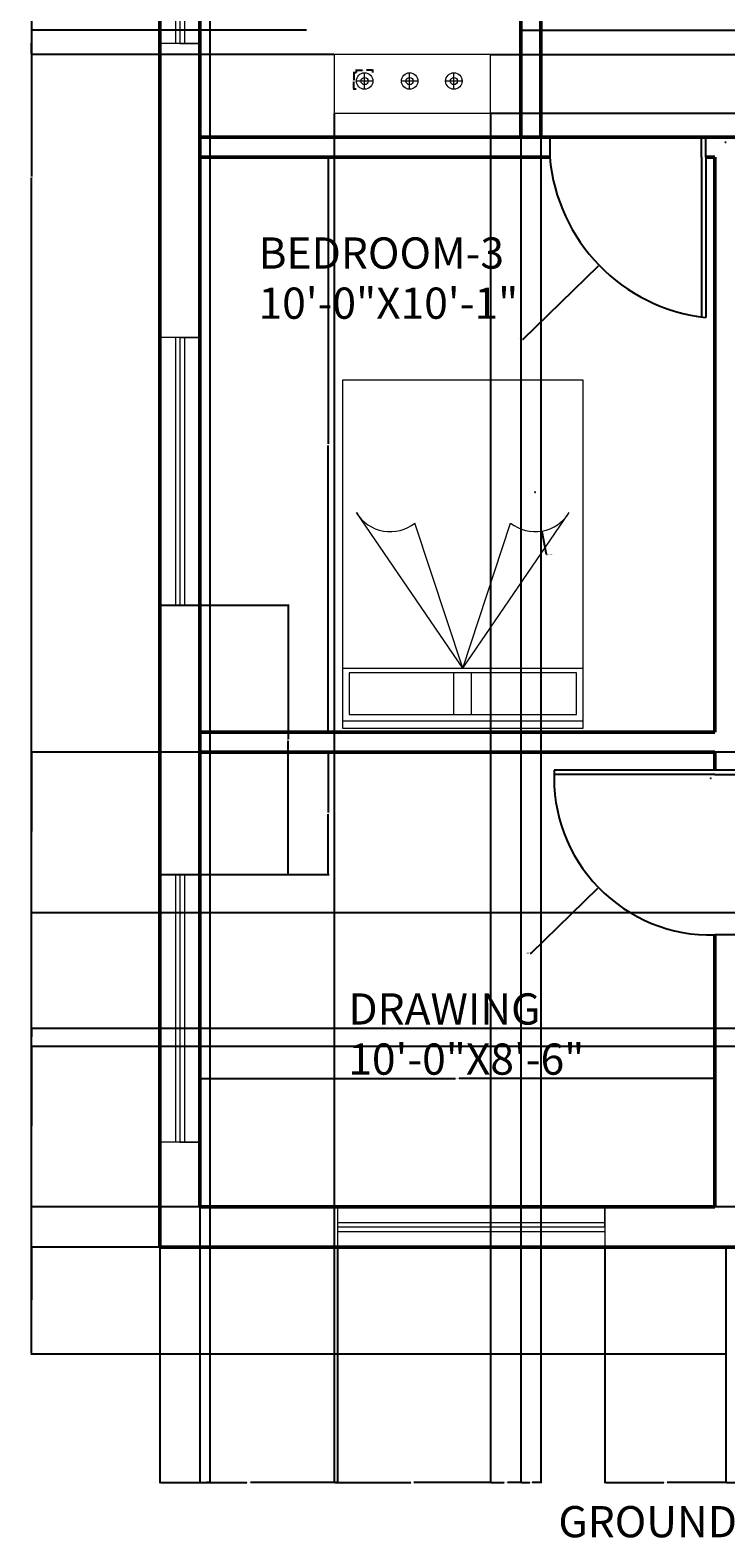
# Model space of a CAD drawing. Units: inches. Extents: x 2750 to 3097, y 1429 to 2028.
# Tile 1 of 4: x 2750 to 2907, y 1429 to 1768. Entities that reach past the tile are written whole.
import ezdxf

# ---------------------------------------------------------------- set-up
doc = ezdxf.new("R2010")
doc.units = ezdxf.units.IN
for name, color, linetype, lineweight in [('A-ANNO-DIMS', 2, 'Continuous', 18), ('A-ANNO-TEXT', 7, 'Continuous', 25), ('A-AREA-IDEN', 7, 'Continuous', 25), ('A-DOOR', 3, 'Continuous', 25), ('A-EQPM', 8, 'Continuous', 18), ('A-FURN', 8, 'Continuous', 18), ('A-GLAZ', 4, 'Continuous', 18), ('A-WALL', 7, 'Continuous', 50)]:
    doc.layers.add(name, color=color, linetype=linetype, lineweight=lineweight)
doc.styles.get("Standard").update_dxf_attribs({"font": 'arial.ttf'})
doc.dimstyles.get("Standard").update_dxf_attribs({"dimtxt": 0.18, "dimasz": 0.18, "dimexe": 0.18, "dimexo": 0.0625, "dimgap": 0.09, "dimtad": 0, "dimtih": 1, "dimtoh": 1, "dimdec": 4, "dimzin": 0, "dimdsep": 46, "dimtxsty": 'Standard', "dimcen": 0.09, "dimadec": 0, "dimazin": 0, "dimtfac": 1, "dimtdec": 4, "dimtofl": 0, "dimtmove": 0, "dimatfit": 3, "dimfxl": 1, "dimtolj": 1, "dimtzin": 0, "dimarcsym": 0})

# ---------------------------------------------------------------- blocks, each defined once
blk = doc.blocks.new('BED-DOUBLE-54X78')
for p, q in [((0, 78), (0, 0)), ((54, 78), (0, 78)), ((54, 0), (54, 78)), ((27, 13.39), (3.13, 48.31)), ((27, 13.39), (50.87, 48.31)), ((27, 13.39), (16.28, 45.98)), ((27, 13.39), (37.72, 45.98)), ((0, 13.39), (54, 13.39)), ((24.99, 3.04), (24.99, 12.35)), ((28.99, 3.04), (28.99, 12.35)), ((0, 1.59), (54, 1.59)), ((0, 0), (54, 0))]:
    blk.add_line(p, q)
blk.add_lwpolyline([(1.48, 3.04), (52.5, 3.04), (52.5, 12.35), (1.48, 12.35)], close=True)
for centre, start, end in [((10.73, 52.93), 211.2898, 308.6091), ((43.27, 52.93), 231.3909, 328.7102)]:
    blk.add_arc(centre, 8.89, start, end)
blk = doc.blocks.new('WIN-60IN')
for p, q in [((9, 60), (0, 60)), ((3.5, 60), (3.5, 0)), ((4.5, 60), (4.5, 0)), ((5.5, 60), (5.5, 0)), ((9, 0), (0, 0))]:
    blk.add_line(p, q)
blk = doc.blocks.new('WIN-36IN')
for p, q in [((9, 36), (0, 36)), ((3.5, 36), (3.5, 0)), ((4.5, 36), (4.5, 0)), ((5.5, 36), (5.5, 0)), ((9, 0), (0, 0))]:
    blk.add_line(p, q)
blk = doc.blocks.new('COOKTOP-BURNER')
for p, q in [((1.85, 0), (1.85, 3.7)), ((3.7, 1.85), (0, 1.85))]:
    blk.add_line(p, q)
for radius in [1.85, 0.81]:
    blk.add_circle((1.85, 1.85), radius)
blk = doc.blocks.new('*D11')
at = {"layer": 'A-ANNO-DIMS', "color": 0, "lineweight": -2, "transparency": 16777216}
for p, q in [((2823.55, 1758), (2822.88, 1758)), ((2823.06, 1757.82), (2823.06, 1756.33)), ((2823.06, 1754.48), (2823.06, 1755.97)), ((2823.55, 1754.3), (2822.88, 1754.3))]:
    blk.add_line(p, q, dxfattribs=at)
at = {"layer": 'A-ANNO-DIMS', "color": 0, "transparency": 16777216}
for points in [[(2823.03, 1757.82), (2823.09, 1757.82), (2823.06, 1758)], [(2823.03, 1754.48), (2823.09, 1754.48), (2823.06, 1754.3)]]:
    blk.add_solid(points, dxfattribs=at)
at = {"layer": 'Defpoints', "color": 0, "transparency": 16777216}
for p in [(2823.06, 1758), (2823.61, 1758), (2823.61, 1754.3)]:
    blk.add_point(p, dxfattribs=at)
at = {"layer": 'A-ANNO-DIMS', "color": 0, "transparency": 16777216, "insert": (2823.06, 1756.15), "char_height": 0.18, "attachment_point": 5}
blk.add_mtext('\\A1;BURNER 4 TYP.', dxfattribs=at)
blk = doc.blocks.new('*D12')
at = {"layer": 'A-ANNO-DIMS', "color": 0, "lineweight": -2, "transparency": 16777216}
for p, q in [((2823.61, 1758.06), (2823.61, 1758.74)), ((2827.31, 1758.06), (2827.31, 1758.74)), ((2823.79, 1758.56), (2825, 1758.56)), ((2827.13, 1758.56), (2825.92, 1758.56))]:
    blk.add_line(p, q, dxfattribs=at)
at = {"layer": 'A-ANNO-DIMS', "color": 0, "transparency": 16777216}
for points in [[(2823.79, 1758.59), (2823.79, 1758.53), (2823.61, 1758.56)], [(2827.13, 1758.59), (2827.13, 1758.53), (2827.31, 1758.56)]]:
    blk.add_solid(points, dxfattribs=at)
at = {"layer": 'Defpoints', "color": 0, "transparency": 16777216}
for p in [(2823.61, 1758), (2827.31, 1758.56), (2827.31, 1758)]:
    blk.add_point(p, dxfattribs=at)
at = {"layer": 'A-ANNO-DIMS', "color": 0, "transparency": 16777216, "insert": (2825.46, 1758.56), "char_height": 0.18, "attachment_point": 5}
blk.add_mtext('\\A1;4 TYP.', dxfattribs=at)
blk = doc.blocks.new('*D14')
at = {"layer": 'A-ANNO-DIMS', "color": 0, "lineweight": -2, "transparency": 16777216}
for p, q in [((2779.46, 1998.59), (2750.54, 1998.59)), ((2750.72, 1998.41), (2750.72, 1734.77)), ((2750.72, 1470.77), (2750.72, 1734.41)), ((2906.46, 1470.59), (2750.54, 1470.59))]:
    blk.add_line(p, q, dxfattribs=at)
at = {"layer": 'A-ANNO-DIMS', "color": 0, "transparency": 16777216}
for points in [[(2750.69, 1998.41), (2750.75, 1998.41), (2750.72, 1998.59)], [(2750.69, 1470.77), (2750.75, 1470.77), (2750.72, 1470.59)]]:
    blk.add_solid(points, dxfattribs=at)
at = {"layer": 'Defpoints', "color": 0, "transparency": 16777216}
for p in [(2750.72, 1998.59), (2779.52, 1998.59), (2906.52, 1470.59)]:
    blk.add_point(p, dxfattribs=at)
at = {"layer": 'A-ANNO-DIMS', "color": 0, "transparency": 16777216, "insert": (2750.72, 1734.59), "char_height": 0.18, "attachment_point": 5}
blk.add_mtext('\\A1;528', dxfattribs=at)
blk = doc.blocks.new('*D15')
at = {"layer": 'A-ANNO-DIMS', "color": 0, "lineweight": -2, "transparency": 16777216}
for p, q in [((2906.46, 1494.59), (2750.54, 1494.59)), ((2750.72, 1494.41), (2750.72, 1482.77)), ((2750.72, 1470.77), (2750.72, 1482.41)), ((2906.46, 1470.59), (2750.54, 1470.59))]:
    blk.add_line(p, q, dxfattribs=at)
at = {"layer": 'A-ANNO-DIMS', "color": 0, "transparency": 16777216}
for points in [[(2750.69, 1494.41), (2750.75, 1494.41), (2750.72, 1494.59)], [(2750.69, 1470.77), (2750.75, 1470.77), (2750.72, 1470.59)]]:
    blk.add_solid(points, dxfattribs=at)
at = {"layer": 'Defpoints', "color": 0, "transparency": 16777216}
for p in [(2750.72, 1494.59), (2906.52, 1494.59), (2906.52, 1470.59)]:
    blk.add_point(p, dxfattribs=at)
at = {"layer": 'A-ANNO-DIMS', "color": 0, "transparency": 16777216, "insert": (2750.72, 1482.59), "char_height": 0.18, "attachment_point": 5}
blk.add_mtext('\\A1;24', dxfattribs=at)
blk = doc.blocks.new('*D16')
at = {"layer": 'A-ANNO-DIMS', "color": 0, "lineweight": -2, "transparency": 16777216}
for p, q in [((2906.52, 1470.53), (2906.52, 1441.61)), ((2955.52, 1470.53), (2955.52, 1441.61)), ((2906.7, 1441.79), (2930.8, 1441.79)), ((2955.34, 1441.79), (2931.24, 1441.79))]:
    blk.add_line(p, q, dxfattribs=at)
at = {"layer": 'A-ANNO-DIMS', "color": 0, "transparency": 16777216}
for points in [[(2906.7, 1441.82), (2906.7, 1441.76), (2906.52, 1441.79)], [(2955.34, 1441.82), (2955.34, 1441.76), (2955.52, 1441.79)]]:
    blk.add_solid(points, dxfattribs=at)
at = {"layer": 'Defpoints', "color": 0, "transparency": 16777216}
for p in [(2906.52, 1470.59), (2955.52, 1470.59), (2955.52, 1441.79)]:
    blk.add_point(p, dxfattribs=at)
at = {"layer": 'A-ANNO-DIMS', "color": 0, "transparency": 16777216, "insert": (2931.02, 1441.79), "char_height": 0.18, "attachment_point": 5}
blk.add_mtext('\\A1;49', dxfattribs=at)
blk = doc.blocks.new('*D17')
at = {"layer": 'A-ANNO-DIMS', "color": 0, "lineweight": -2, "transparency": 16777216}
for p, q in [((2779.52, 1494.53), (2779.52, 1441.61)), ((2819.4, 1494.53), (2819.4, 1441.61)), ((2779.7, 1441.79), (2799.07, 1441.79)), ((2819.22, 1441.79), (2799.85, 1441.79))]:
    blk.add_line(p, q, dxfattribs=at)
at = {"layer": 'A-ANNO-DIMS', "color": 0, "transparency": 16777216}
for points in [[(2779.7, 1441.82), (2779.7, 1441.76), (2779.52, 1441.79)], [(2819.22, 1441.82), (2819.22, 1441.76), (2819.4, 1441.79)]]:
    blk.add_solid(points, dxfattribs=at)
at = {"layer": 'Defpoints', "color": 0, "transparency": 16777216}
for p in [(2779.52, 1494.59), (2819.4, 1494.59), (2819.4, 1441.79)]:
    blk.add_point(p, dxfattribs=at)
at = {"layer": 'A-ANNO-DIMS', "color": 0, "transparency": 16777216, "insert": (2799.46, 1441.79), "char_height": 0.18, "attachment_point": 5}
blk.add_mtext('\\A1;39.88', dxfattribs=at)
blk = doc.blocks.new('*D18')
at = {"layer": 'A-ANNO-DIMS', "color": 0, "lineweight": -2, "transparency": 16777216}
for p, q in [((2879.4, 1494.53), (2879.4, 1441.61)), ((2906.52, 1494.53), (2906.52, 1441.61)), ((2879.58, 1441.79), (2892.57, 1441.79)), ((2906.34, 1441.79), (2893.36, 1441.79))]:
    blk.add_line(p, q, dxfattribs=at)
at = {"layer": 'A-ANNO-DIMS', "color": 0, "transparency": 16777216}
for points in [[(2879.58, 1441.82), (2879.58, 1441.76), (2879.4, 1441.79)], [(2906.34, 1441.82), (2906.34, 1441.76), (2906.52, 1441.79)]]:
    blk.add_solid(points, dxfattribs=at)
at = {"layer": 'Defpoints', "color": 0, "transparency": 16777216}
for p in [(2879.4, 1494.59), (2906.52, 1494.59), (2906.52, 1441.79)]:
    blk.add_point(p, dxfattribs=at)
at = {"layer": 'A-ANNO-DIMS', "color": 0, "transparency": 16777216, "insert": (2892.96, 1441.79), "char_height": 0.18, "attachment_point": 5}
blk.add_mtext('\\A1;27.12', dxfattribs=at)
blk = doc.blocks.new('*D20')
at = {"layer": 'A-ANNO-DIMS', "color": 0, "lineweight": -2, "transparency": 16777216}
for p, q in [((2788.58, 1605.59), (2817.5, 1605.59)), ((2817.32, 1605.41), (2817.32, 1592.05)), ((2817.32, 1578.32), (2817.32, 1591.68)), ((2788.58, 1578.14), (2817.5, 1578.14))]:
    blk.add_line(p, q, dxfattribs=at)
at = {"layer": 'A-ANNO-DIMS', "color": 0, "transparency": 16777216}
for points in [[(2817.29, 1605.41), (2817.35, 1605.41), (2817.32, 1605.59)], [(2817.29, 1578.32), (2817.35, 1578.32), (2817.32, 1578.14)]]:
    blk.add_solid(points, dxfattribs=at)
at = {"layer": 'Defpoints', "color": 0, "transparency": 16777216}
for p in [(2788.52, 1605.59), (2788.52, 1578.14), (2817.32, 1578.14)]:
    blk.add_point(p, dxfattribs=at)
at = {"layer": 'A-ANNO-DIMS', "color": 0, "transparency": 16777216, "insert": (2817.32, 1591.86), "char_height": 0.18, "attachment_point": 5}
blk.add_mtext('\\A1;27.457', dxfattribs=at)
blk = doc.blocks.new('*D21')
at = {"layer": 'A-ANNO-DIMS', "color": 0, "lineweight": -2, "transparency": 16777216}
for p, q in [((2779.58, 1638.59), (2808.5, 1638.59)), ((2808.32, 1638.41), (2808.32, 1608.55)), ((2808.32, 1578.32), (2808.32, 1608.18)), ((2779.58, 1578.14), (2808.5, 1578.14))]:
    blk.add_line(p, q, dxfattribs=at)
at = {"layer": 'A-ANNO-DIMS', "color": 0, "transparency": 16777216}
for points in [[(2808.29, 1638.41), (2808.35, 1638.41), (2808.32, 1638.59)], [(2808.29, 1578.32), (2808.35, 1578.32), (2808.32, 1578.14)]]:
    blk.add_solid(points, dxfattribs=at)
at = {"layer": 'Defpoints', "color": 0, "transparency": 16777216}
for p in [(2779.52, 1638.59), (2779.52, 1578.14), (2808.32, 1578.14)]:
    blk.add_point(p, dxfattribs=at)
at = {"layer": 'A-ANNO-DIMS', "color": 0, "transparency": 16777216, "insert": (2808.32, 1608.36), "char_height": 0.18, "attachment_point": 5}
blk.add_mtext('\\A1;60.46', dxfattribs=at)
blk = doc.blocks.new('*D31')
at = {"layer": 'A-ANNO-DIMS', "color": 0, "lineweight": -2, "transparency": 16777216}
for p, q in [((2788.58, 1739.09), (2817.5, 1739.09)), ((2817.32, 1738.91), (2817.32, 1674.77)), ((2817.32, 1610.27), (2817.32, 1674.41)), ((2788.58, 1610.09), (2817.5, 1610.09))]:
    blk.add_line(p, q, dxfattribs=at)
at = {"layer": 'A-ANNO-DIMS', "color": 0, "transparency": 16777216}
for points in [[(2817.29, 1738.91), (2817.35, 1738.91), (2817.32, 1739.09)], [(2817.29, 1610.27), (2817.35, 1610.27), (2817.32, 1610.09)]]:
    blk.add_solid(points, dxfattribs=at)
at = {"layer": 'Defpoints', "color": 0, "transparency": 16777216}
for p in [(2788.52, 1739.09), (2788.52, 1610.09), (2817.32, 1610.09)]:
    blk.add_point(p, dxfattribs=at)
at = {"layer": 'A-ANNO-DIMS', "color": 0, "transparency": 16777216, "insert": (2817.32, 1674.59), "char_height": 0.18, "attachment_point": 5}
blk.add_mtext('\\A1;129', dxfattribs=at)
blk = doc.blocks.new('*D32')
at = {"layer": 'A-ANNO-DIMS', "color": 0, "lineweight": -2, "transparency": 16777216}
for p, q in [((2788.52, 1503.66), (2788.52, 1532.57)), ((2788.7, 1532.39), (2845.88, 1532.39)), ((2903.84, 1532.39), (2846.66, 1532.39)), ((2904.02, 1503.66), (2904.02, 1532.57))]:
    blk.add_line(p, q, dxfattribs=at)
at = {"layer": 'A-ANNO-DIMS', "color": 0, "transparency": 16777216}
for points in [[(2788.7, 1532.42), (2788.7, 1532.36), (2788.52, 1532.39)], [(2903.84, 1532.42), (2903.84, 1532.36), (2904.02, 1532.39)]]:
    blk.add_solid(points, dxfattribs=at)
at = {"layer": 'Defpoints', "color": 0, "transparency": 16777216}
for p in [(2904.02, 1532.39), (2788.52, 1503.59), (2904.02, 1503.59)]:
    blk.add_point(p, dxfattribs=at)
at = {"layer": 'A-ANNO-DIMS', "color": 0, "transparency": 16777216, "insert": (2846.27, 1532.39), "char_height": 0.18, "attachment_point": 5}
blk.add_mtext('\\A1;115.5', dxfattribs=at)
blk = doc.blocks.new('*D39')
at = {"layer": 'A-ANNO-DIMS', "color": 0, "lineweight": -2, "transparency": 16777216}
for p, q in [((2860.58, 1767.56), (3096.5, 1767.56)), ((3096.32, 1767.38), (3096.32, 1755.76)), ((3096.32, 1743.77), (3096.32, 1755.4)), ((2860.58, 1743.59), (3096.5, 1743.59))]:
    blk.add_line(p, q, dxfattribs=at)
at = {"layer": 'A-ANNO-DIMS', "color": 0, "transparency": 16777216}
for points in [[(3096.29, 1767.38), (3096.35, 1767.38), (3096.32, 1767.56)], [(3096.29, 1743.77), (3096.35, 1743.77), (3096.32, 1743.59)]]:
    blk.add_solid(points, dxfattribs=at)
at = {"layer": 'Defpoints', "color": 0, "transparency": 16777216}
for p in [(2860.52, 1767.56), (3096.32, 1767.56), (2860.52, 1743.59)]:
    blk.add_point(p, dxfattribs=at)
at = {"layer": 'A-ANNO-DIMS', "color": 0, "transparency": 16777216, "insert": (3096.32, 1755.58), "char_height": 0.18, "attachment_point": 5}
blk.add_mtext('\\A1;23.97', dxfattribs=at)
blk = doc.blocks.new('*D42')
at = {"layer": 'A-ANNO-DIMS', "color": 0, "lineweight": -2, "transparency": 16777216}
for p, q in [((2860.52, 1797.53), (2860.52, 1441.61)), ((2865.02, 1797.53), (2865.02, 1441.61)), ((2860.7, 1441.79), (2862.51, 1441.79)), ((2864.84, 1441.79), (2863.03, 1441.79))]:
    blk.add_line(p, q, dxfattribs=at)
at = {"layer": 'A-ANNO-DIMS', "color": 0, "transparency": 16777216}
for points in [[(2860.7, 1441.82), (2860.7, 1441.76), (2860.52, 1441.79)], [(2864.84, 1441.82), (2864.84, 1441.76), (2865.02, 1441.79)]]:
    blk.add_solid(points, dxfattribs=at)
at = {"layer": 'Defpoints', "color": 0, "transparency": 16777216}
for p in [(2860.52, 1797.59), (2865.02, 1797.59), (2865.02, 1441.79)]:
    blk.add_point(p, dxfattribs=at)
at = {"layer": 'A-ANNO-DIMS', "color": 0, "transparency": 16777216, "insert": (2862.77, 1441.79), "char_height": 0.18, "attachment_point": 5}
blk.add_mtext('\\A1;4.5', dxfattribs=at)
blk = doc.blocks.new('*D46')
at = {"layer": 'A-ANNO-DIMS', "color": 0, "lineweight": -2, "transparency": 16777216}
for p, q in [((2790.76, 1771.54), (2790.76, 1441.61)), ((2788.52, 1764.53), (2788.52, 1441.61)), ((2788.7, 1441.79), (2789.32, 1441.79)), ((2790.58, 1441.79), (2789.97, 1441.79))]:
    blk.add_line(p, q, dxfattribs=at)
at = {"layer": 'A-ANNO-DIMS', "color": 0, "transparency": 16777216}
for points in [[(2788.7, 1441.82), (2788.7, 1441.76), (2788.52, 1441.79)], [(2790.58, 1441.82), (2790.58, 1441.76), (2790.76, 1441.79)]]:
    blk.add_solid(points, dxfattribs=at)
at = {"layer": 'Defpoints', "color": 0, "transparency": 16777216}
for p in [(2790.76, 1771.61), (2788.52, 1764.59), (2790.76, 1441.79)]:
    blk.add_point(p, dxfattribs=at)
at = {"layer": 'A-ANNO-DIMS', "color": 0, "transparency": 16777216, "insert": (2789.64, 1441.79), "char_height": 0.18, "attachment_point": 5}
blk.add_mtext('\\A1;2.24', dxfattribs=at)
blk = doc.blocks.new('*D47')
at = {"layer": 'A-ANNO-DIMS', "color": 0, "lineweight": -2, "transparency": 16777216}
for p, q in [((2818.61, 1748.9), (2818.61, 1441.61)), ((2853.71, 1748.9), (2853.71, 1441.61)), ((2818.79, 1441.79), (2835.85, 1441.79)), ((2853.53, 1441.79), (2836.47, 1441.79))]:
    blk.add_line(p, q, dxfattribs=at)
at = {"layer": 'A-ANNO-DIMS', "color": 0, "transparency": 16777216}
for points in [[(2818.79, 1441.82), (2818.79, 1441.76), (2818.61, 1441.79)], [(2853.53, 1441.82), (2853.53, 1441.76), (2853.71, 1441.79)]]:
    blk.add_solid(points, dxfattribs=at)
at = {"layer": 'Defpoints', "color": 0, "transparency": 16777216}
for p in [(2818.61, 1748.96), (2853.71, 1748.96), (2853.71, 1441.79)]:
    blk.add_point(p, dxfattribs=at)
at = {"layer": 'A-ANNO-DIMS', "color": 0, "transparency": 16777216, "insert": (2836.16, 1441.79), "char_height": 0.18, "attachment_point": 5}
blk.add_mtext('\\A1;35.1', dxfattribs=at)
blk = doc.blocks.new('*D48')
at = {"layer": 'A-ANNO-DIMS', "color": 0, "lineweight": -2, "transparency": 16777216}
for p, q in [((2853.77, 1762.1), (3096.5, 1762.1)), ((3096.32, 1761.92), (3096.32, 1755.71)), ((3096.32, 1749.14), (3096.32, 1755.35)), ((2853.77, 1748.96), (3096.5, 1748.96))]:
    blk.add_line(p, q, dxfattribs=at)
at = {"layer": 'A-ANNO-DIMS', "color": 0, "transparency": 16777216}
for points in [[(3096.29, 1761.92), (3096.35, 1761.92), (3096.32, 1762.1)], [(3096.29, 1749.14), (3096.35, 1749.14), (3096.32, 1748.96)]]:
    blk.add_solid(points, dxfattribs=at)
at = {"layer": 'Defpoints', "color": 0, "transparency": 16777216}
for p in [(2853.71, 1762.1), (3096.32, 1762.1), (2853.71, 1748.96)]:
    blk.add_point(p, dxfattribs=at)
at = {"layer": 'A-ANNO-DIMS', "color": 0, "transparency": 16777216, "insert": (3096.32, 1755.53), "char_height": 0.18, "attachment_point": 5}
blk.add_mtext('\\A1;13.143', dxfattribs=at)
blk = doc.blocks.new('*D49')
at = {"layer": 'A-ANNO-DIMS', "color": 0, "lineweight": -2, "transparency": 16777216}
for p, q in [((2853.71, 1748.9), (2853.71, 1441.61)), ((2860.52, 1743.53), (2860.52, 1441.61)), ((2853.89, 1441.79), (2856.74, 1441.79)), ((2860.34, 1441.79), (2857.49, 1441.79))]:
    blk.add_line(p, q, dxfattribs=at)
at = {"layer": 'A-ANNO-DIMS', "color": 0, "transparency": 16777216}
for points in [[(2853.89, 1441.82), (2853.89, 1441.76), (2853.71, 1441.79)], [(2860.34, 1441.82), (2860.34, 1441.76), (2860.52, 1441.79)]]:
    blk.add_solid(points, dxfattribs=at)
at = {"layer": 'Defpoints', "color": 0, "transparency": 16777216}
for p in [(2853.71, 1748.96), (2860.52, 1743.59), (2860.52, 1441.79)]:
    blk.add_point(p, dxfattribs=at)
at = {"layer": 'A-ANNO-DIMS', "color": 0, "transparency": 16777216, "insert": (2857.11, 1441.79), "char_height": 0.18, "attachment_point": 5}
blk.add_mtext('\\A1;6.811', dxfattribs=at)
blk = doc.blocks.new('*D50')
at = {"layer": 'A-ANNO-DIMS', "color": 0, "lineweight": -2, "transparency": 16777216}
for p, q in [((2812.46, 1767.56), (2750.54, 1767.56)), ((2750.72, 1767.38), (2750.72, 1765.01)), ((2818.55, 1762.1), (2750.54, 1762.1)), ((2750.72, 1762.28), (2750.72, 1764.65))]:
    blk.add_line(p, q, dxfattribs=at)
at = {"layer": 'A-ANNO-DIMS', "color": 0, "transparency": 16777216}
for points in [[(2750.69, 1767.38), (2750.75, 1767.38), (2750.72, 1767.56)], [(2750.69, 1762.28), (2750.75, 1762.28), (2750.72, 1762.1)]]:
    blk.add_solid(points, dxfattribs=at)
at = {"layer": 'Defpoints', "color": 0, "transparency": 16777216}
for p in [(2750.72, 1767.56), (2812.52, 1767.56), (2818.61, 1762.1)]:
    blk.add_point(p, dxfattribs=at)
at = {"layer": 'A-ANNO-DIMS', "color": 0, "transparency": 16777216, "insert": (2750.72, 1764.83), "char_height": 0.18, "attachment_point": 5}
blk.add_mtext('\\A1;5.461', dxfattribs=at)
blk = doc.blocks.new('*D54')
at = {"layer": 'A-ANNO-DIMS', "color": 0, "lineweight": -2, "transparency": 16777216}
for p, q in [((2972.46, 1605.59), (2750.54, 1605.59)), ((2750.72, 1605.41), (2750.72, 1587.77)), ((2750.72, 1569.77), (2750.72, 1587.41)), ((2972.46, 1569.59), (2750.54, 1569.59))]:
    blk.add_line(p, q, dxfattribs=at)
at = {"layer": 'A-ANNO-DIMS', "color": 0, "transparency": 16777216}
for points in [[(2750.69, 1605.41), (2750.75, 1605.41), (2750.72, 1605.59)], [(2750.69, 1569.77), (2750.75, 1569.77), (2750.72, 1569.59)]]:
    blk.add_solid(points, dxfattribs=at)
at = {"layer": 'Defpoints', "color": 0, "transparency": 16777216}
for p in [(2750.72, 1605.59), (2972.52, 1605.59), (2972.52, 1569.59)]:
    blk.add_point(p, dxfattribs=at)
at = {"layer": 'A-ANNO-DIMS', "color": 0, "transparency": 16777216, "insert": (2750.72, 1587.59), "char_height": 0.18, "attachment_point": 5}
blk.add_mtext('\\A1;36', dxfattribs=at)
blk = doc.blocks.new('*D56')
at = {"layer": 'A-ANNO-DIMS', "color": 0, "lineweight": -2, "transparency": 16777216}
for p, q in [((2996.46, 1539.59), (2750.54, 1539.59)), ((2750.72, 1539.41), (2750.72, 1521.77)), ((2750.72, 1503.77), (2750.72, 1521.41)), ((2996.46, 1503.59), (2750.54, 1503.59))]:
    blk.add_line(p, q, dxfattribs=at)
at = {"layer": 'A-ANNO-DIMS', "color": 0, "transparency": 16777216}
for points in [[(2750.69, 1539.41), (2750.75, 1539.41), (2750.72, 1539.59)], [(2750.69, 1503.77), (2750.75, 1503.77), (2750.72, 1503.59)]]:
    blk.add_solid(points, dxfattribs=at)
at = {"layer": 'Defpoints', "color": 0, "transparency": 16777216}
for p in [(2750.72, 1539.59), (2996.52, 1539.59), (2996.52, 1503.59)]:
    blk.add_point(p, dxfattribs=at)
at = {"layer": 'A-ANNO-DIMS', "color": 0, "transparency": 16777216, "insert": (2750.72, 1521.59), "char_height": 0.18, "attachment_point": 5}
blk.add_mtext('\\A1;36', dxfattribs=at)
blk = doc.blocks.new('*D57')
at = {"layer": 'A-ANNO-DIMS', "color": 0, "lineweight": -2, "transparency": 16777216}
for p, q in [((2996.457604, 1543.592536), (2750.540104, 1543.592536)), ((2750.720104, 1543.412536), (2750.720104, 1541.772536)), ((2996.457604, 1539.592536), (2750.540104, 1539.592536)), ((2750.720104, 1539.772536), (2750.720104, 1541.412536))]:
    blk.add_line(p, q, dxfattribs=at)
at = {"layer": 'A-ANNO-DIMS', "color": 0, "transparency": 16777216}
for points in [[(2750.690104, 1543.412536), (2750.750104, 1543.412536), (2750.720104, 1543.592536)], [(2750.690104, 1539.772536), (2750.750104, 1539.772536), (2750.720104, 1539.592536)]]:
    blk.add_solid(points, dxfattribs=at)
at = {"layer": 'Defpoints', "color": 0, "transparency": 16777216}
for p in [(2750.720104, 1543.592536), (2996.520104, 1543.592536), (2996.520104, 1539.592536)]:
    blk.add_point(p, dxfattribs=at)
at = {"layer": 'A-ANNO-DIMS', "color": 0, "transparency": 16777216, "insert": (2750.720104, 1541.592536), "char_height": 0.18, "attachment_point": 5}
blk.add_mtext('\\A1;4', dxfattribs=at)
blk = doc.blocks.new('*D61')
at = {"layer": 'A-ANNO-DIMS', "color": 0, "lineweight": -2, "transparency": 16777216}
for p, q in [((2906.38, 1742.43), (2906.56, 1742.43)), ((2906.47, 1742.34), (2906.47, 1742.52)), ((2861.05, 1698.28), (2877.95, 1714.71)), ((2860.87, 1698.28), (2861.05, 1698.28))]:
    blk.add_line(p, q, dxfattribs=at)
at = {"layer": 'A-ANNO-DIMS', "color": 0, "transparency": 16777216}
blk.add_solid([(2877.93, 1714.73), (2877.98, 1714.69), (2878.08, 1714.83)], dxfattribs=at)
at = {"layer": 'Defpoints', "color": 0, "transparency": 16777216}
for p in [(2906.47, 1742.43), (2878.08, 1714.83)]:
    blk.add_point(p, dxfattribs=at)
at = {"layer": 'A-ANNO-DIMS', "color": 0, "transparency": 16777216, "insert": (2860.39, 1698.28), "char_height": 0.18, "attachment_point": 5}
blk.add_mtext('\\A1;R39.59', dxfattribs=at)
blk = doc.blocks.new('*D63')
at = {"layer": 'A-ANNO-DIMS', "color": 0, "lineweight": -2, "transparency": 16777216}
for p, q in [((2903.06, 1599.76), (2903.24, 1599.76)), ((2903.15, 1599.67), (2903.15, 1599.85)), ((2862.81, 1560.51), (2877.81, 1575.1)), ((2862.63, 1560.51), (2862.81, 1560.51))]:
    blk.add_line(p, q, dxfattribs=at)
at = {"layer": 'A-ANNO-DIMS', "color": 0, "transparency": 16777216}
blk.add_solid([(2877.79, 1575.13), (2877.83, 1575.08), (2877.94, 1575.23)], dxfattribs=at)
at = {"layer": 'Defpoints', "color": 0, "transparency": 16777216}
for p in [(2903.15, 1599.76), (2877.94, 1575.23)]:
    blk.add_point(p, dxfattribs=at)
at = {"layer": 'A-ANNO-DIMS', "color": 0, "transparency": 16777216, "insert": (2862.15, 1560.51), "char_height": 0.18, "attachment_point": 5}
blk.add_mtext('\\A1;R35.18', dxfattribs=at)
blk = doc.blocks.new('*D66')
at = {"layer": 'A-ANNO-DIMS', "color": 0, "lineweight": -2, "transparency": 16777216}
for p, q in [((2863.75, 1663.86), (2863.75, 1664.04)), ((2863.66, 1663.95), (2863.84, 1663.95)), ((2866.24, 1649.93), (2865.34, 1655.01)), ((2866.42, 1649.93), (2866.24, 1649.93))]:
    blk.add_line(p, q, dxfattribs=at)
at = {"layer": 'A-ANNO-DIMS', "color": 0, "transparency": 16777216}
blk.add_solid([(2865.37, 1655.02), (2865.31, 1655.01), (2865.31, 1655.19)], dxfattribs=at)
at = {"layer": 'Defpoints', "color": 0, "transparency": 16777216}
for p in [(2863.75, 1663.95), (2865.31, 1655.19)]:
    blk.add_point(p, dxfattribs=at)
at = {"layer": 'A-ANNO-DIMS', "color": 0, "transparency": 16777216, "insert": (2867.09, 1649.93), "char_height": 0.18, "attachment_point": 5}
blk.add_mtext('\\A1;6X R8.894', dxfattribs=at)

msp = doc.modelspace()

# ---------------------------------------------------------------- linework, layer by layer
at = {"layer": 'A-DOOR'}
for p, q in [((2867.0201, 1743.5925), (2867.0201, 1739.0925)), ((2901.0204, 1739.0566), (2901.0204, 1743.5925)), ((2902.0204, 1739.0566), (2902.0204, 1743.5925)), ((2901.0204, 1739.0925), (2901.0204, 1703.2186)), ((2902.0204, 1739.0925), (2902.0204, 1703.0925)), ((2904.0201, 1601.5926), (2868.0201, 1601.5926)), ((2904.0201, 1600.5926), (2868.0201, 1600.5926)), ((2908.534, 1601.5926), (2904.0201, 1601.5926)), ((2904.0201, 1600.5926), (2908.5201, 1600.5926)), ((2908.5201, 1564.5926), (2904.0201, 1564.5926))]:
    msp.add_line(p, q, dxfattribs=at)
for centre, radius, start, end in [((2906.4716, 1742.4343), 39.5928, 184.841733, 263.544936), ((2903.1533, 1599.7627), 35.1808, 177.018469, 271.411882)]:
    msp.add_arc(centre, radius, start, end, dxfattribs=at)
at = {"layer": 'A-EQPM'}
msp.add_lwpolyline([(2818.609, 1748.9592), (2853.7089, 1748.9592), (2853.7089, 1762.1022), (2818.609, 1762.1022)], close=True, dxfattribs=at)
at = {"layer": 'A-GLAZ'}
for p, q in [((2784.0201, 1764.5925), (2788.5201, 1764.5925)), ((2784.0201, 1764.5925), (2784.0201, 1764.5925)), ((2784.0201, 1698.5925), (2788.5201, 1698.5925)), ((2784.0201, 1638.5925), (2788.5201, 1638.5925)), ((2784.0201, 1578.1359), (2784.0201, 1518.1359)), ((2785.0201, 1578.1359), (2785.0201, 1518.1359)), ((2784.0201, 1571.5925), (2784.0201, 1571.5925)), ((2784.0201, 1518.1359), (2788.5201, 1518.1359)), ((2879.4017, 1499.0925), (2879.4017, 1503.5925))]:
    msp.add_line(p, q, dxfattribs=at)
at = {"layer": 'A-WALL'}
for p, q in [((2779.5201, 1494.5925), (2779.5201, 1998.5925)), ((2788.5201, 1503.5925), (2788.5201, 1989.5925)), ((2860.5201, 1743.5925), (2860.5201, 1773.5925)), ((2865.0201, 1743.5925), (2865.0201, 1773.5925)), ((2788.5201, 1743.5925), (2908.5201, 1743.5925)), ((2865.0201, 1743.5925), (2867.0201, 1743.5925)), ((2788.5201, 1739.0925), (2867.0201, 1739.0925)), ((2902.0204, 1739.0925), (2904.0201, 1739.0925)), ((2904.0201, 1610.0925), (2904.0201, 1739.0925)), ((2904.0201, 1610.0925), (2788.5201, 1610.0925)), ((2904.0201, 1605.5925), (2788.5201, 1605.5925)), ((2904.0201, 1601.5926), (2904.0201, 1605.5925)), ((2904.0201, 1503.5925), (2904.0201, 1564.5926)), ((2904.0201, 1503.5925), (2788.5201, 1503.5925)), ((3067.5201, 1494.5925), (2779.5201, 1494.5925))]:
    msp.add_line(p, q, dxfattribs=at)

# ---------------------------------------------------------------- block references
at = {"layer": 'A-EQPM'}
for p in [(2823.6117, 1754.301), (2833.7179, 1754.301), (2843.648, 1754.301)]:
    msp.add_blockref('COOKTOP-BURNER', p, dxfattribs=at)
at = {"layer": 'A-FURN'}
msp.add_blockref('BED-DOUBLE-54X78', (2820.486, 1611.018), dxfattribs=at)
at = {"layer": 'A-GLAZ'}
for name, p in [('WIN-36IN', (2779.52, 1764.593)), ('WIN-60IN', (2779.52, 1638.593)), ('WIN-60IN', (2779.52, 1518.1363))]:
    msp.add_blockref(name, p, dxfattribs=at)
at = {"layer": 'A-GLAZ', "rotation": 90.00000000000126}
msp.add_blockref('WIN-60IN', (2879.4013, 1494.5924), dxfattribs=at)

# ---------------------------------------------------------------- texts
at = {"layer": 'A-ANNO-TEXT'}
msp.add_text('GROUND FLOOR PLAN', height=7, dxfattribs=at).set_placement((2868.9383, 1429.4831))
at = {"layer": 'A-AREA-IDEN'}
for s, p in [('BEDROOM-3', (2801.669, 1714.0666)), ('10\'-0"X10\'-1"', (2801.669, 1702.8218)), ('DRAWING', (2821.8077, 1544.4994)), ('10\'-0"X8\'-6"', (2821.8077, 1533.2545))]:
    msp.add_text(s, height=7, dxfattribs=at).set_placement(p)

# ---------------------------------------------------------------- dimensions: what is measured, and where the dimension line sits
at = {"layer": 'A-ANNO-DIMS'}
for base, p1, p2, angle, override, picture, middle in [((2750.7201, 1998.5925), (2906.5201, 1470.5925), (2779.5201, 1998.5925), 90, {"dimdec": 0, "dimlfac": 1, "dimrnd": 0, "dimzin": 0, "dimdsep": 46, "dimlunit": 2}, '*D14', (2750.7201, 1734.5925)), ((2750.7201, 1767.5629), (2818.609, 1762.1022), (2812.5201, 1767.5629), 90, {"dimdec": 3, "dimlfac": 1, "dimrnd": 0, "dimzin": 0, "dimdsep": 46, "dimlunit": 2}, '*D50', (2750.7201, 1764.8326)), ((3096.3201, 1767.5629), (2860.5201, 1743.5925), (2860.5201, 1767.5629), 90, {"dimdec": 2, "dimlfac": 1, "dimrnd": 0, "dimzin": 0, "dimdsep": 46, "dimlunit": 2}, '*D39', (3096.3201, 1755.5777)), ((3096.3201, 1762.1022), (2853.7089, 1748.9592), (2853.7089, 1762.1022), 90, {"dimdec": 3, "dimlfac": 1, "dimrnd": 0, "dimzin": 0, "dimdsep": 46, "dimlunit": 2}, '*D48', (3096.3201, 1755.5307)), ((2817.3201, 1610.0925), (2788.5201, 1739.0925), (2788.5201, 1610.0925), 270, {"dimdec": 0, "dimlfac": 1, "dimrnd": 0, "dimzin": 0, "dimdsep": 46, "dimlunit": 2}, '*D31', (2817.3201, 1674.5925)), ((2808.3201, 1578.1359), (2779.5201, 1638.5925), (2779.5201, 1578.1359), 270, {"dimdec": 2, "dimlfac": 1, "dimrnd": 0, "dimzin": 0, "dimdsep": 46, "dimlunit": 2}, '*D21', (2808.3201, 1608.3642)), ((2750.7201, 1605.5925), (2972.5201, 1569.5925), (2972.5201, 1605.5925), 90, {"dimdec": 0, "dimlfac": 1, "dimrnd": 0, "dimzin": 0, "dimdsep": 46, "dimlunit": 2}, '*D54', (2750.7201, 1587.5925)), ((2817.3201, 1578.1359), (2788.5201, 1605.5925), (2788.5201, 1578.1359), 270, {"dimdec": 3, "dimlfac": 1, "dimrnd": 0, "dimzin": 0, "dimdsep": 46, "dimlunit": 2}, '*D20', (2817.3201, 1591.8642)), ((2750.7201, 1543.5925), (2996.5201, 1539.5925), (2996.5201, 1543.5925), 90, {"dimdec": 0, "dimlfac": 1, "dimrnd": 0, "dimzin": 0, "dimdsep": 46, "dimlunit": 2}, '*D57', (2750.7201, 1541.5925)), ((2750.7201, 1539.5925), (2996.5201, 1503.5925), (2996.5201, 1539.5925), 90, {"dimdec": 0, "dimlfac": 1, "dimrnd": 0, "dimzin": 0, "dimdsep": 46, "dimlunit": 2}, '*D56', (2750.7201, 1521.5925)), ((2750.7201, 1494.5925), (2906.5201, 1470.5925), (2906.5201, 1494.5925), 90, {"dimdec": 0, "dimlfac": 1, "dimrnd": 0, "dimzin": 0, "dimdsep": 46, "dimlunit": 2}, '*D15', (2750.7201, 1482.5925))]:
    dim = msp.add_linear_dim(base=base, p1=p1, p2=p2, angle=angle, dimstyle='Standard', override=override, dxfattribs=at)
    dim.commit()
    dim.dimension.update_dxf_attribs({"geometry": picture, "text_midpoint": middle})
for base, p1, p2, override, picture, middle in [((2865.0201, 1441.7925), (2860.5201, 1797.5925), (2865.0201, 1797.5925), {"dimdec": 1, "dimlfac": 1, "dimrnd": 0, "dimzin": 0, "dimdsep": 46, "dimlunit": 2}, '*D42', (2862.7701, 1441.7925)), ((2790.7618, 1441.7925), (2788.5201, 1764.5925), (2790.7618, 1771.6062), {"dimdec": 2, "dimlfac": 1, "dimrnd": 0, "dimzin": 0, "dimdsep": 46, "dimlunit": 2}, '*D46', (2789.641, 1441.7925)), ((2853.7089, 1441.7925), (2818.609, 1748.9592), (2853.7089, 1748.9592), {"dimdec": 1, "dimlfac": 1, "dimrnd": 0, "dimzin": 0, "dimdsep": 46, "dimlunit": 2}, '*D47', (2836.159, 1441.7925)), ((2860.5201, 1441.7925), (2853.7089, 1748.9592), (2860.5201, 1743.5925), {"dimdec": 3, "dimlfac": 1, "dimrnd": 0, "dimzin": 0, "dimdsep": 46, "dimlunit": 2}, '*D49', (2857.1145, 1441.7925)), ((2904.0201, 1532.3925), (2788.5201, 1503.5925), (2904.0201, 1503.5925), {"dimdec": 1, "dimlfac": 1, "dimrnd": 0, "dimzin": 0, "dimdsep": 46, "dimlunit": 2}, '*D32', (2846.2701, 1532.3925)), ((2819.4017, 1441.7925), (2779.5201, 1494.5925), (2819.4017, 1494.5925), {"dimdec": 2, "dimlfac": 1, "dimrnd": 0, "dimzin": 0, "dimdsep": 46, "dimlunit": 2}, '*D17', (2799.4609, 1441.7925)), ((2906.5201, 1441.7925), (2879.4017, 1494.5925), (2906.5201, 1494.5925), {"dimdec": 2, "dimlfac": 1, "dimrnd": 0, "dimzin": 0, "dimdsep": 46, "dimlunit": 2}, '*D18', (2892.9609, 1441.7925)), ((2955.5201, 1441.7925), (2906.5201, 1470.5925), (2955.5201, 1470.5925), {"dimdec": 0, "dimlfac": 1, "dimrnd": 0, "dimzin": 0, "dimdsep": 46, "dimlunit": 2}, '*D16', (2931.0201, 1441.7925))]:
    dim = msp.add_linear_dim(base=base, p1=p1, p2=p2, dimstyle='Standard', override=override, dxfattribs=at)
    dim.commit()
    dim.dimension.update_dxf_attribs({"geometry": picture, "text_midpoint": middle})
dim = msp.add_linear_dim(base=(2827.3132, 1758.5577), p1=(2823.6118, 1758.0025), p2=(2827.3132, 1758.0025), text='<> TYP.', dimstyle='Standard', override={"dimdec": 0, "dimlfac": 1, "dimrnd": 0, "dimzin": 0, "dimdsep": 46, "dimlunit": 2}, dxfattribs=at)
dim.commit()
dim.dimension.update_dxf_attribs({"geometry": '*D12', "text_midpoint": (2825.4625, 1758.5577)})
dim = msp.add_linear_dim(base=(2823.0565, 1758.0025), p1=(2823.6118, 1754.301), p2=(2823.6118, 1758.0025), angle=90, text='BURNER <> TYP.', dimstyle='Standard', override={"dimdec": 0, "dimlfac": 1, "dimrnd": 0, "dimzin": 0, "dimdsep": 46, "dimlunit": 2}, dxfattribs=at)
dim.commit()
dim.dimension.update_dxf_attribs({"geometry": '*D11', "text_midpoint": (2823.0565, 1756.1517)})
for center, mpoint, picture, middle in [((2906.4716, 1742.4343), (2878.0839, 1714.8349), '*D61', (2860.3913, 1698.2753)), ((2903.1533, 1599.7627), (2877.9382, 1575.2292), '*D63', (2862.1492, 1560.5092))]:
    dim = msp.add_radius_dim(center=center, mpoint=mpoint, dimstyle='Standard', override={"dimdec": 2, "dimlfac": 1, "dimrnd": 0, "dimzin": 0, "dimdsep": 46, "dimlunit": 2}, dxfattribs=at)
    dim.commit()
    dim.dimension.update_dxf_attribs({"geometry": picture, "text_midpoint": middle, "dimtype": 164})
dim = msp.add_radius_dim(center=(2863.7524, 1663.9464), mpoint=(2865.305, 1655.1889), text='6X <>', dimstyle='Standard', override={"dimdec": 3, "dimlfac": 1, "dimrnd": 0, "dimzin": 0, "dimdsep": 46, "dimlunit": 2}, dxfattribs=at)
dim.commit()
dim.dimension.update_dxf_attribs({"geometry": '*D66', "text_midpoint": (2867.0899, 1649.9344), "dimtype": 164})

doc.saveas('drawing.dxf')
